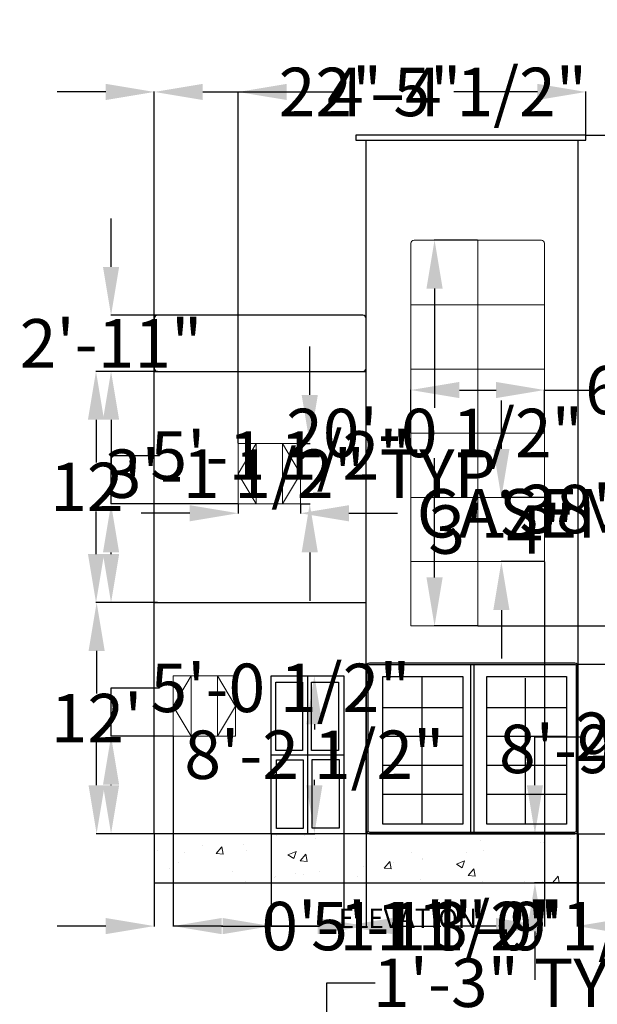
# Model space of a CAD drawing. Units: inches. Extents: x 7323 to 9737, y 2037 to 3322.
# Tile 17 of 19: x 8562 to 8922, y 2709 to 3322. Entities that reach past the tile are written whole.
import ezdxf

# ---------------------------------------------------------------- set-up
doc = ezdxf.new("R2010")
doc.units = ezdxf.units.IN
doc.header["$MEASUREMENT"] = 0
for name, color, linetype, lineweight in [('A-ANNO-DIMS', 2, 'Continuous', 18), ('A-ANNO-TEXT', 7, 'Continuous', 25), ('A-DOOR', 4, 'Continuous', 25), ('A-ELEV', 7, 'Continuous', 30), ('A-GLAZ', 4, 'Continuous', 18), ('A-ROOF', 7, 'Continuous', 30)]:
    doc.layers.add(name, color=color, linetype=linetype, lineweight=lineweight)
doc.layers.add('A-ELEV-PATT', color=32, linetype='Continuous', lineweight=13, true_color=0xcd6928)
doc.styles.get("Standard").update_dxf_attribs({"font": 'arial.ttf'})
doc.dimstyles.get("Standard").update_dxf_attribs({"dimtxt": 30.18, "dimasz": 30.18, "dimexe": 0.18, "dimexo": 0.0625, "dimgap": 0.09, "dimtad": 0, "dimtih": 1, "dimtoh": 1, "dimdec": 0, "dimzin": 0, "dimdsep": 46, "dimlunit": 3, "dimtxsty": 'Standard', "dimcen": 0.09, "dimadec": 0, "dimazin": 0, "dimtfac": 1, "dimtdec": 0, "dimtofl": 0, "dimtmove": 0, "dimatfit": 3, "dimfxl": 1, "dimtolj": 1, "dimtzin": 0, "dimarcsym": 0})

# ---------------------------------------------------------------- blocks, each defined once
blk = doc.blocks.new('*D5')
at = {"layer": 'A-ANNO-DIMS', "color": 0, "lineweight": -2, "transparency": 16777216}
for p, q in [((8646.01, 2959.19), (8610, 2959.19)), ((8610.18, 2929.01), (8610.18, 2902.43)), ((8610.18, 2845.37), (8610.18, 2871.95)), ((8646.01, 2815.19), (8610, 2815.19))]:
    blk.add_line(p, q, dxfattribs=at)
at = {"layer": 'A-ANNO-DIMS', "color": 0, "transparency": 16777216}
for points in [[(8605.15, 2929.01), (8615.21, 2929.01), (8610.18, 2959.19)], [(8605.15, 2845.37), (8615.21, 2845.37), (8610.18, 2815.19)]]:
    blk.add_solid(points, dxfattribs=at)
at = {"layer": 'Defpoints', "color": 0, "transparency": 16777216}
for p in [(8610.18, 2959.19), (8646.07, 2959.19), (8646.07, 2815.19)]:
    blk.add_point(p, dxfattribs=at)
at = {"layer": 'A-ANNO-DIMS', "color": 0, "transparency": 16777216, "insert": (8610.18, 2887.19), "char_height": 30.18, "attachment_point": 5}
blk.add_mtext("\\A1;12'", dxfattribs=at)
blk = doc.blocks.new('*D6')
at = {"layer": 'A-ANNO-DIMS', "color": 0, "lineweight": -2, "transparency": 16777216}
for p, q in [((8648.01, 3103.19), (8609.62, 3103.19)), ((8609.8, 3073.01), (8609.8, 3046.43)), ((8609.8, 2989.37), (8609.8, 3015.95)), ((8648.01, 2959.19), (8609.62, 2959.19))]:
    blk.add_line(p, q, dxfattribs=at)
at = {"layer": 'A-ANNO-DIMS', "color": 0, "transparency": 16777216}
for points in [[(8604.77, 3073.01), (8614.83, 3073.01), (8609.8, 3103.19)], [(8604.77, 2989.37), (8614.83, 2989.37), (8609.8, 2959.19)]]:
    blk.add_solid(points, dxfattribs=at)
at = {"layer": 'Defpoints', "color": 0, "transparency": 16777216}
for p in [(8648.07, 3103.19), (8609.8, 2959.19), (8648.07, 2959.19)]:
    blk.add_point(p, dxfattribs=at)
at = {"layer": 'A-ANNO-DIMS', "color": 0, "transparency": 16777216, "insert": (8609.8, 3031.19), "char_height": 30.18, "attachment_point": 5}
blk.add_mtext("\\A1;12'", dxfattribs=at)
blk = doc.blocks.new('WIN-ELEV-CASEMENT')
for p, q in [((11.18, 37.71), (0, 18.85)), ((11.18, 37.71), (11.18, 0)), ((27.64, 37.71), (27.64, 0)), ((27.64, 37.71), (38.77, 18.85)), ((0, 18.85), (11.18, 0)), ((38.77, 18.85), (27.64, 0))]:
    blk.add_line(p, q)
blk.add_lwpolyline([(38.77, 37.71), (38.77, 37.71), (0, 37.71), (0, 37.71), (0, 0), (0, 0), (38.77, 0), (38.77, 0)], close=True)
blk = doc.blocks.new('*D45')
at = {"layer": 'A-ANNO-DIMS', "color": 0, "lineweight": -2, "transparency": 16777216}
for p, q in [((8725.79, 2664.36), (8695.61, 2664.36)), ((8755.97, 2662.02), (8755.97, 2664.54)), ((8772, 2662.02), (8772, 2664.54)), ((8802.18, 2664.36), (8832.36, 2664.36))]:
    blk.add_line(p, q, dxfattribs=at)
at = {"layer": 'A-ANNO-DIMS', "color": 0, "transparency": 16777216}
for points in [[(8725.79, 2669.39), (8725.79, 2659.33), (8755.97, 2664.36)], [(8802.18, 2669.39), (8802.18, 2659.33), (8772, 2664.36)]]:
    blk.add_solid(points, dxfattribs=at)
at = {"layer": 'Defpoints', "color": 0, "transparency": 16777216}
for p in [(8755.97, 2661.96), (8772, 2664.36), (8772, 2661.96)]:
    blk.add_point(p, dxfattribs=at)
at = {"layer": 'A-ANNO-DIMS', "color": 0, "transparency": 16777216, "insert": (9094.8, 2664.36), "char_height": 30.18, "attachment_point": 5}
blk.add_mtext('\\A1;BEDSIDE TABLE 1\'-4" TYP.', dxfattribs=at)
blk = doc.blocks.new('*D46')
at = {"layer": 'A-ANNO-DIMS', "color": 0, "lineweight": -2, "transparency": 16777216}
for p, q in [((8753.57, 2692.14), (8753.57, 2722.32)), ((8753.57, 2722.32), (8783.75, 2722.32)), ((8755.91, 2661.96), (8753.39, 2661.96)), ((8755.91, 2647.12), (8753.39, 2647.12)), ((8753.57, 2616.94), (8753.57, 2586.76))]:
    blk.add_line(p, q, dxfattribs=at)
at = {"layer": 'A-ANNO-DIMS', "color": 0, "transparency": 16777216}
for points in [[(8748.54, 2692.14), (8758.6, 2692.14), (8753.57, 2661.96)], [(8748.54, 2616.94), (8758.6, 2616.94), (8753.57, 2647.12)]]:
    blk.add_solid(points, dxfattribs=at)
at = {"layer": 'Defpoints', "color": 0, "transparency": 16777216}
for p in [(8753.57, 2661.96), (8755.97, 2661.96), (8755.97, 2647.12)]:
    blk.add_point(p, dxfattribs=at)
at = {"layer": 'A-ANNO-DIMS', "color": 0, "transparency": 16777216, "insert": (8874.4, 2722.32), "char_height": 30.18, "attachment_point": 5}
blk.add_mtext('\\A1;1\'-3" TYP.', dxfattribs=at)
blk = doc.blocks.new('*D57')
at = {"layer": 'A-ANNO-DIMS', "color": 0, "lineweight": -2, "transparency": 16777216}
for p, q in [((8698.34, 3020.54), (8698.34, 3014.6)), ((8737.11, 3020.54), (8737.11, 3014.6)), ((8668.16, 3014.78), (8637.98, 3014.78)), ((8767.29, 3014.78), (8797.47, 3014.78))]:
    blk.add_line(p, q, dxfattribs=at)
at = {"layer": 'A-ANNO-DIMS', "color": 0, "transparency": 16777216}
for points in [[(8668.16, 3019.81), (8668.16, 3009.75), (8698.34, 3014.78)], [(8767.29, 3019.81), (8767.29, 3009.75), (8737.11, 3014.78)]]:
    blk.add_solid(points, dxfattribs=at)
at = {"layer": 'Defpoints', "color": 0, "transparency": 16777216}
for p in [(8698.34, 3020.6), (8737.11, 3020.6), (8737.11, 3014.78)]:
    blk.add_point(p, dxfattribs=at)
at = {"layer": 'A-ANNO-DIMS', "color": 0, "transparency": 16777216, "insert": (9012.35, 3014.78), "char_height": 30.18, "attachment_point": 5}
blk.add_mtext('\\A1;CASEMENT 3\'-3" TYP.', dxfattribs=at)
blk = doc.blocks.new('*D58')
at = {"layer": 'A-ANNO-DIMS', "color": 0, "lineweight": -2, "transparency": 16777216}
for p, q in [((8742.92, 3088.49), (8742.92, 3118.67)), ((8737.17, 3058.31), (8743.1, 3058.31)), ((8737.17, 3020.6), (8743.1, 3020.6)), ((8742.92, 2990.42), (8742.92, 2960.24))]:
    blk.add_line(p, q, dxfattribs=at)
at = {"layer": 'A-ANNO-DIMS', "color": 0, "transparency": 16777216}
for points in [[(8737.89, 3088.49), (8747.95, 3088.49), (8742.92, 3058.31)], [(8737.89, 2990.42), (8747.95, 2990.42), (8742.92, 3020.6)]]:
    blk.add_solid(points, dxfattribs=at)
at = {"layer": 'Defpoints', "color": 0, "transparency": 16777216}
for p in [(8737.11, 3058.31), (8742.92, 3058.31), (8737.11, 3020.6)]:
    blk.add_point(p, dxfattribs=at)
at = {"layer": 'A-ANNO-DIMS', "color": 0, "transparency": 16777216, "insert": (8742.92, 3039.45), "char_height": 30.18, "attachment_point": 5}
blk.add_mtext('\\A1;3\'-1 1/2" TYP.', dxfattribs=at)
blk = doc.blocks.new('*D82')
at = {"layer": 'A-ANNO-DIMS', "color": 0, "lineweight": -2, "transparency": 16777216}
for p, q in [((8646.07, 3103.25), (8646.07, 3277.41)), ((8676.25, 3277.23), (8728.3, 3277.23)), ((8884.72, 3277.23), (8832.67, 3277.23)), ((8914.9, 3250.4), (8914.9, 3277.41))]:
    blk.add_line(p, q, dxfattribs=at)
at = {"layer": 'A-ANNO-DIMS', "color": 0, "transparency": 16777216}
for points in [[(8676.25, 3282.26), (8676.25, 3272.2), (8646.07, 3277.23)], [(8884.72, 3282.26), (8884.72, 3272.2), (8914.9, 3277.23)]]:
    blk.add_solid(points, dxfattribs=at)
at = {"layer": 'Defpoints', "color": 0, "transparency": 16777216}
for p in [(8914.9, 3277.23), (8914.9, 3250.33), (8646.07, 3103.19)]:
    blk.add_point(p, dxfattribs=at)
at = {"layer": 'A-ANNO-DIMS', "color": 0, "transparency": 16777216, "insert": (8780.48, 3277.23), "char_height": 30.18, "attachment_point": 5}
blk.add_mtext('\\A1;22\'-5"', dxfattribs=at)
blk = doc.blocks.new('*D83')
at = {"layer": 'A-ANNO-DIMS', "color": 0, "lineweight": -2, "transparency": 16777216}
for p, q in [((8914.96, 3250.33), (8941.98, 3250.33)), ((8941.8, 3220.15), (8941.8, 3032.95)), ((8941.8, 2814.72), (8941.8, 3001.93)), ((8910.13, 2784.54), (8941.98, 2784.54))]:
    blk.add_line(p, q, dxfattribs=at)
at = {"layer": 'A-ANNO-DIMS', "color": 0, "transparency": 16777216}
for points in [[(8936.77, 3220.15), (8946.83, 3220.15), (8941.8, 3250.33)], [(8936.77, 2814.72), (8946.83, 2814.72), (8941.8, 2784.54)]]:
    blk.add_solid(points, dxfattribs=at)
at = {"layer": 'Defpoints', "color": 0, "transparency": 16777216}
for p in [(8914.9, 3250.33), (8941.8, 3250.33), (8910.07, 2784.54)]:
    blk.add_point(p, dxfattribs=at)
at = {"layer": 'A-ANNO-DIMS', "color": 0, "transparency": 16777216, "insert": (8941.8, 3017.44), "char_height": 30.18, "attachment_point": 5}
blk.add_mtext('\\A1;38\'-10"', dxfattribs=at)
blk = doc.blocks.new('*D84')
at = {"layer": 'A-ANNO-DIMS', "color": 0, "lineweight": -2, "transparency": 16777216}
for p, q in [((8778.071366, 2815.126036), (8778.071366, 2757.459848)), ((8910.071366, 2815.126036), (8910.071366, 2757.459848)), ((8747.891366, 2757.639848), (8717.711366, 2757.639848)), ((8940.251366, 2757.639848), (8970.431366, 2757.639848))]:
    blk.add_line(p, q, dxfattribs=at)
at = {"layer": 'A-ANNO-DIMS', "color": 0, "transparency": 16777216}
for points in [[(8747.891366, 2762.669848), (8747.891366, 2752.609848), (8778.071366, 2757.639848)], [(8940.251366, 2762.669848), (8940.251366, 2752.609848), (8910.071366, 2757.639848)]]:
    blk.add_solid(points, dxfattribs=at)
at = {"layer": 'Defpoints', "color": 0, "transparency": 16777216}
for p in [(8778.071366, 2815.188536), (8910.071366, 2815.188536), (8910.071366, 2757.639848)]:
    blk.add_point(p, dxfattribs=at)
at = {"layer": 'A-ANNO-DIMS', "color": 0, "transparency": 16777216, "insert": (8844.071366, 2757.639848), "char_height": 30.18, "attachment_point": 5}
blk.add_mtext('\\A1;11\'-0"', dxfattribs=at)
blk = doc.blocks.new('*D85')
at = {"layer": 'A-ANNO-DIMS', "color": 0, "lineweight": -2, "transparency": 16777216}
for p, q in [((8805.94, 3064.71), (8805.94, 3091.73)), ((8836.12, 3091.55), (8858.99, 3091.55)), ((8889.17, 3064.71), (8889.17, 3091.73)), ((8889.17, 3091.55), (8919.35, 3091.55))]:
    blk.add_line(p, q, dxfattribs=at)
at = {"layer": 'A-ANNO-DIMS', "color": 0, "transparency": 16777216}
for points in [[(8836.12, 3096.58), (8836.12, 3086.52), (8805.94, 3091.55)], [(8858.99, 3096.58), (8858.99, 3086.52), (8889.17, 3091.55)]]:
    blk.add_solid(points, dxfattribs=at)
at = {"layer": 'Defpoints', "color": 0, "transparency": 16777216}
for p in [(8889.17, 3091.55), (8805.94, 3064.65), (8889.17, 3064.65)]:
    blk.add_point(p, dxfattribs=at)
at = {"layer": 'A-ANNO-DIMS', "color": 0, "transparency": 16777216, "insert": (8971.36, 3091.55), "char_height": 30.18, "attachment_point": 5}
blk.add_mtext('\\A1;6\'-11"', dxfattribs=at)
blk = doc.blocks.new('*D86')
at = {"layer": 'A-ANNO-DIMS', "color": 0, "lineweight": -2, "transparency": 16777216}
for p, q in [((8847.49, 3184.93), (8820.47, 3184.93)), ((8820.65, 3154.75), (8820.65, 3080.48)), ((8820.65, 2974.83), (8820.65, 3049.09)), ((8847.49, 2944.65), (8820.47, 2944.65))]:
    blk.add_line(p, q, dxfattribs=at)
at = {"layer": 'A-ANNO-DIMS', "color": 0, "transparency": 16777216}
for points in [[(8815.62, 3154.75), (8825.68, 3154.75), (8820.65, 3184.93)], [(8815.62, 2974.83), (8825.68, 2974.83), (8820.65, 2944.65)]]:
    blk.add_solid(points, dxfattribs=at)
at = {"layer": 'Defpoints', "color": 0, "transparency": 16777216}
for p in [(8820.65, 3184.93), (8847.55, 3184.93), (8847.55, 2944.65)]:
    blk.add_point(p, dxfattribs=at)
at = {"layer": 'A-ANNO-DIMS', "color": 0, "transparency": 16777216, "insert": (8820.65, 3064.79), "char_height": 30.18, "attachment_point": 5}
blk.add_mtext('\\A1;20\'-0 1/2"', dxfattribs=at)
blk = doc.blocks.new('*D87')
at = {"layer": 'A-ANNO-DIMS', "color": 0, "lineweight": -2, "transparency": 16777216}
for p, q in [((8619.17, 2875.84), (8619.17, 2906.02)), ((8619.17, 2906.02), (8649.35, 2906.02)), ((8657.74, 2875.84), (8618.99, 2875.84)), ((8619.17, 2845.37), (8619.17, 2845.66)), ((8646.01, 2815.19), (8618.99, 2815.19))]:
    blk.add_line(p, q, dxfattribs=at)
at = {"layer": 'A-ANNO-DIMS', "color": 0, "transparency": 16777216}
for points in [[(8614.14, 2845.66), (8624.2, 2845.66), (8619.17, 2875.84)], [(8614.14, 2845.37), (8624.2, 2845.37), (8619.17, 2815.19)]]:
    blk.add_solid(points, dxfattribs=at)
at = {"layer": 'Defpoints', "color": 0, "transparency": 16777216}
for p in [(8619.17, 2875.84), (8657.81, 2875.84), (8646.07, 2815.19)]:
    blk.add_point(p, dxfattribs=at)
at = {"layer": 'A-ANNO-DIMS', "color": 0, "transparency": 16777216, "insert": (8724.72, 2906.02), "char_height": 30.18, "attachment_point": 5}
blk.add_mtext('\\A1;5\'-0 1/2"', dxfattribs=at)
blk = doc.blocks.new('*D88')
at = {"layer": 'A-ANNO-DIMS', "color": 0, "lineweight": -2, "transparency": 16777216}
for p, q in [((8941.797746, 2974.828285), (8941.797746, 3005.008285)), ((8941.797746, 3005.008285), (8971.977746, 3005.008285)), ((8847.615005, 2944.648285), (8941.977746, 2944.648285)), ((8909.54808, 2920.815964), (8941.977746, 2920.815964)), ((8941.797746, 2890.635964), (8941.797746, 2860.455964))]:
    blk.add_line(p, q, dxfattribs=at)
at = {"layer": 'A-ANNO-DIMS', "color": 0, "transparency": 16777216}
for points in [[(8936.767746, 2974.828285), (8946.827746, 2974.828285), (8941.797746, 2944.648285)], [(8936.767746, 2890.635964), (8946.827746, 2890.635964), (8941.797746, 2920.815964)]]:
    blk.add_solid(points, dxfattribs=at)
at = {"layer": 'Defpoints', "color": 0, "transparency": 16777216}
for p in [(8847.552505, 2944.648285), (8941.797746, 2944.648285), (8909.48558, 2920.815964)]:
    blk.add_point(p, dxfattribs=at)
at = {"layer": 'A-ANNO-DIMS', "color": 0, "transparency": 16777216, "insert": (9012.438128, 3005.008285), "char_height": 30.18, "attachment_point": 5}
blk.add_mtext('\\A1;2\'-0"', dxfattribs=at)
blk = doc.blocks.new('*D89')
at = {"layer": 'A-ANNO-DIMS', "color": 0, "lineweight": -2, "transparency": 16777216}
for p, q in [((8657.81, 2875.78), (8657.81, 2757.46)), ((8718.91, 2815.13), (8718.91, 2757.46)), ((8687.99, 2757.64), (8688.73, 2757.64)), ((8718.91, 2757.64), (8749.09, 2757.64))]:
    blk.add_line(p, q, dxfattribs=at)
at = {"layer": 'A-ANNO-DIMS', "color": 0, "transparency": 16777216}
for points in [[(8687.99, 2762.67), (8687.99, 2752.61), (8657.81, 2757.64)], [(8688.73, 2762.67), (8688.73, 2752.61), (8718.91, 2757.64)]]:
    blk.add_solid(points, dxfattribs=at)
at = {"layer": 'Defpoints', "color": 0, "transparency": 16777216}
for p in [(8657.81, 2875.84), (8718.91, 2815.19), (8718.91, 2757.64)]:
    blk.add_point(p, dxfattribs=at)
at = {"layer": 'A-ANNO-DIMS', "color": 0, "transparency": 16777216, "insert": (8789.29, 2757.64), "char_height": 30.18, "attachment_point": 5}
blk.add_mtext('\\A1;5\'-1"', dxfattribs=at)
blk = doc.blocks.new('*D90')
at = {"layer": 'A-ANNO-DIMS', "color": 0, "lineweight": -2, "transparency": 16777216}
for p, q in [((8718.91, 2815.13), (8718.91, 2757.46)), ((8764.24, 2815.13), (8764.24, 2757.46)), ((8688.73, 2757.64), (8658.55, 2757.64)), ((8794.42, 2757.64), (8824.6, 2757.64))]:
    blk.add_line(p, q, dxfattribs=at)
at = {"layer": 'A-ANNO-DIMS', "color": 0, "transparency": 16777216}
for points in [[(8688.73, 2762.67), (8688.73, 2752.61), (8718.91, 2757.64)], [(8794.42, 2762.67), (8794.42, 2752.61), (8764.24, 2757.64)]]:
    blk.add_solid(points, dxfattribs=at)
at = {"layer": 'Defpoints', "color": 0, "transparency": 16777216}
for p in [(8718.91, 2815.19), (8764.24, 2815.19), (8764.24, 2757.64)]:
    blk.add_point(p, dxfattribs=at)
at = {"layer": 'A-ANNO-DIMS', "color": 0, "transparency": 16777216, "insert": (8899.95, 2757.64), "char_height": 30.18, "attachment_point": 5}
blk.add_mtext('\\A1;3\'-9 1/2"', dxfattribs=at)
blk = doc.blocks.new('*D91')
at = {"layer": 'A-ANNO-DIMS', "color": 0, "lineweight": -2, "transparency": 16777216}
for p, q in [((8909.55, 2920.82), (8941.98, 2920.82)), ((8941.8, 2890.64), (8941.8, 2883.7)), ((8941.8, 2845.37), (8941.8, 2852.31)), ((8910.13, 2815.19), (8941.98, 2815.19))]:
    blk.add_line(p, q, dxfattribs=at)
at = {"layer": 'A-ANNO-DIMS', "color": 0, "transparency": 16777216}
for points in [[(8936.77, 2890.64), (8946.83, 2890.64), (8941.8, 2920.82)], [(8936.77, 2845.37), (8946.83, 2845.37), (8941.8, 2815.19)]]:
    blk.add_solid(points, dxfattribs=at)
at = {"layer": 'Defpoints', "color": 0, "transparency": 16777216}
for p in [(8909.49, 2920.82), (8941.8, 2920.82), (8910.07, 2815.19)]:
    blk.add_point(p, dxfattribs=at)
at = {"layer": 'A-ANNO-DIMS', "color": 0, "transparency": 16777216, "insert": (8941.8, 2868), "char_height": 30.18, "attachment_point": 5}
blk.add_mtext('\\A1;8\'-9 1/2"', dxfattribs=at)
blk = doc.blocks.new('*D92')
at = {"layer": 'A-ANNO-DIMS', "color": 0, "lineweight": -2, "transparency": 16777216}
for p, q in [((8883.17, 2845.37), (8883.17, 2875.55)), ((8883.17, 2875.55), (8913.35, 2875.55)), ((8910.01, 2815.19), (8882.99, 2815.19)), ((8910.01, 2784.54), (8882.99, 2784.54)), ((8883.17, 2754.36), (8883.17, 2724.18))]:
    blk.add_line(p, q, dxfattribs=at)
at = {"layer": 'A-ANNO-DIMS', "color": 0, "transparency": 16777216}
for points in [[(8878.14, 2845.37), (8888.2, 2845.37), (8883.17, 2815.19)], [(8878.14, 2754.36), (8888.2, 2754.36), (8883.17, 2784.54)]]:
    blk.add_solid(points, dxfattribs=at)
at = {"layer": 'Defpoints', "color": 0, "transparency": 16777216}
for p in [(8883.17, 2815.19), (8910.07, 2815.19), (8910.07, 2784.54)]:
    blk.add_point(p, dxfattribs=at)
at = {"layer": 'A-ANNO-DIMS', "color": 0, "transparency": 16777216, "insert": (8988.97, 2875.55), "char_height": 30.18, "attachment_point": 5}
blk.add_mtext('\\A1;2\'-6 1/2"', dxfattribs=at)
blk = doc.blocks.new('*D101')
at = {"layer": 'A-ANNO-DIMS', "color": 0, "lineweight": -2, "transparency": 16777216}
for p, q in [((8889.17, 2984.59), (8889.17, 2757.46)), ((8909.49, 2920.75), (8909.49, 2757.46)), ((8858.99, 2757.64), (8828.81, 2757.64)), ((8939.67, 2757.64), (8969.85, 2757.64))]:
    blk.add_line(p, q, dxfattribs=at)
at = {"layer": 'A-ANNO-DIMS', "color": 0, "transparency": 16777216}
for points in [[(8858.99, 2762.67), (8858.99, 2752.61), (8889.17, 2757.64)], [(8939.67, 2762.67), (8939.67, 2752.61), (8909.49, 2757.64)]]:
    blk.add_solid(points, dxfattribs=at)
at = {"layer": 'Defpoints', "color": 0, "transparency": 16777216}
for p in [(8889.17, 2984.65), (8909.49, 2920.82), (8909.49, 2757.64)]:
    blk.add_point(p, dxfattribs=at)
at = {"layer": 'A-ANNO-DIMS', "color": 0, "transparency": 16777216, "insert": (9043.79, 2757.64), "char_height": 30.18, "attachment_point": 5}
blk.add_mtext('\\A1;1\'-8 1/2"', dxfattribs=at)
blk = doc.blocks.new('*D102')
at = {"layer": 'A-ANNO-DIMS', "color": 0, "lineweight": -2, "transparency": 16777216}
for p, q in [((8619.171366, 3168.286532), (8619.171366, 3198.466532)), ((8648.008866, 3138.106532), (8618.991366, 3138.106532)), ((8646.008866, 3103.188536), (8618.991366, 3103.188536)), ((8619.171366, 3073.008536), (8619.171366, 3042.828536))]:
    blk.add_line(p, q, dxfattribs=at)
at = {"layer": 'A-ANNO-DIMS', "color": 0, "transparency": 16777216}
for points in [[(8614.141366, 3168.286532), (8624.201366, 3168.286532), (8619.171366, 3138.106532)], [(8614.141366, 3073.008536), (8624.201366, 3073.008536), (8619.171366, 3103.188536)]]:
    blk.add_solid(points, dxfattribs=at)
at = {"layer": 'Defpoints', "color": 0, "transparency": 16777216}
for p in [(8619.171366, 3138.106532), (8648.071366, 3138.106532), (8646.071366, 3103.188536)]:
    blk.add_point(p, dxfattribs=at)
at = {"layer": 'A-ANNO-DIMS', "color": 0, "transparency": 16777216, "insert": (8619.171366, 3120.647534), "char_height": 30.18, "attachment_point": 5}
blk.add_mtext('\\A1;2\'-11"', dxfattribs=at)
blk = doc.blocks.new('*D117')
at = {"layer": 'A-ANNO-DIMS', "color": 0, "lineweight": -2, "transparency": 16777216}
for p, q in [((8862.269216, 3054.828285), (8862.269216, 3085.008285)), ((8889.106716, 3024.648285), (8862.089216, 3024.648285)), ((8889.106716, 2984.648285), (8862.089216, 2984.648285)), ((8862.269216, 2954.468285), (8862.269216, 2924.288285))]:
    blk.add_line(p, q, dxfattribs=at)
at = {"layer": 'A-ANNO-DIMS', "color": 0, "transparency": 16777216}
for points in [[(8857.239216, 3054.828285), (8867.299216, 3054.828285), (8862.269216, 3024.648285)], [(8857.239216, 2954.468285), (8867.299216, 2954.468285), (8862.269216, 2984.648285)]]:
    blk.add_solid(points, dxfattribs=at)
at = {"layer": 'Defpoints', "color": 0, "transparency": 16777216}
for p in [(8862.269216, 3024.648285), (8889.169216, 3024.648285), (8889.169216, 2984.648285)]:
    blk.add_point(p, dxfattribs=at)
at = {"layer": 'A-ANNO-DIMS', "color": 0, "transparency": 16777216, "insert": (8862.269216, 3004.648285), "char_height": 30.18, "attachment_point": 5}
blk.add_mtext('\\A1;3\'-4"', dxfattribs=at)
blk = doc.blocks.new('*D118')
at = {"layer": 'A-ANNO-DIMS', "color": 0, "lineweight": -2, "transparency": 16777216}
for p, q in [((8718.97, 2913.55), (8745.99, 2913.55)), ((8745.81, 2883.37), (8745.81, 2880.06)), ((8745.81, 2845.37), (8745.81, 2848.67)), ((8718.97, 2815.19), (8745.99, 2815.19))]:
    blk.add_line(p, q, dxfattribs=at)
at = {"layer": 'A-ANNO-DIMS', "color": 0, "transparency": 16777216}
for points in [[(8740.78, 2883.37), (8750.84, 2883.37), (8745.81, 2913.55)], [(8740.78, 2845.37), (8750.84, 2845.37), (8745.81, 2815.19)]]:
    blk.add_solid(points, dxfattribs=at)
at = {"layer": 'Defpoints', "color": 0, "transparency": 16777216}
for p in [(8718.91, 2913.55), (8718.91, 2815.19), (8745.81, 2815.19)]:
    blk.add_point(p, dxfattribs=at)
at = {"layer": 'A-ANNO-DIMS', "color": 0, "transparency": 16777216, "insert": (8745.81, 2864.37), "char_height": 30.18, "attachment_point": 5}
blk.add_mtext('\\A1;8\'-2 1/2"', dxfattribs=at)
blk = doc.blocks.new('*D119')
at = {"layer": 'A-ANNO-DIMS', "color": 0, "lineweight": -2, "transparency": 16777216}
for p, q in [((8619.17, 3020.6), (8619.17, 3050.78)), ((8619.17, 3050.78), (8649.35, 3050.78)), ((8698.27, 3020.6), (8618.99, 3020.6)), ((8619.17, 2989.37), (8619.17, 2990.42)), ((8646.01, 2959.19), (8618.99, 2959.19))]:
    blk.add_line(p, q, dxfattribs=at)
at = {"layer": 'A-ANNO-DIMS', "color": 0, "transparency": 16777216}
for points in [[(8614.14, 2990.42), (8624.2, 2990.42), (8619.17, 3020.6)], [(8614.14, 2989.37), (8624.2, 2989.37), (8619.17, 2959.19)]]:
    blk.add_solid(points, dxfattribs=at)
at = {"layer": 'Defpoints', "color": 0, "transparency": 16777216}
for p in [(8619.17, 3020.6), (8698.34, 3020.6), (8646.07, 2959.19)]:
    blk.add_point(p, dxfattribs=at)
at = {"layer": 'A-ANNO-DIMS', "color": 0, "transparency": 16777216, "insert": (8724.72, 3050.78), "char_height": 30.18, "attachment_point": 5}
blk.add_mtext('\\A1;5\'-1 1/2"', dxfattribs=at)
blk = doc.blocks.new('*D120')
at = {"layer": 'A-ANNO-DIMS', "color": 0, "lineweight": -2, "transparency": 16777216}
for p, q in [((8615.89, 3277.23), (8585.71, 3277.23)), ((8646.07, 3103.25), (8646.07, 3277.41)), ((8698.34, 3058.37), (8698.34, 3277.41)), ((8728.52, 3277.23), (8758.7, 3277.23))]:
    blk.add_line(p, q, dxfattribs=at)
at = {"layer": 'A-ANNO-DIMS', "color": 0, "transparency": 16777216}
for points in [[(8615.89, 3282.26), (8615.89, 3272.2), (8646.07, 3277.23)], [(8728.52, 3282.26), (8728.52, 3272.2), (8698.34, 3277.23)]]:
    blk.add_solid(points, dxfattribs=at)
at = {"layer": 'Defpoints', "color": 0, "transparency": 16777216}
for p in [(8698.34, 3277.23), (8646.07, 3103.19), (8698.34, 3058.31)]:
    blk.add_point(p, dxfattribs=at)
at = {"layer": 'A-ANNO-DIMS', "color": 0, "transparency": 16777216, "insert": (8834.67, 3277.23), "char_height": 30.18, "attachment_point": 5}
blk.add_mtext('\\A1;4\'-4 1/2"', dxfattribs=at)
blk = doc.blocks.new('*D121')
at = {"layer": 'A-ANNO-DIMS', "color": 0, "lineweight": -2, "transparency": 16777216}
for p, q in [((8657.81, 2875.78), (8657.81, 2757.46)), ((8646.07, 2815.13), (8646.07, 2757.46)), ((8615.89, 2757.64), (8585.71, 2757.64)), ((8687.99, 2757.64), (8718.17, 2757.64))]:
    blk.add_line(p, q, dxfattribs=at)
at = {"layer": 'A-ANNO-DIMS', "color": 0, "transparency": 16777216}
for points in [[(8615.89, 2762.67), (8615.89, 2752.61), (8646.07, 2757.64)], [(8687.99, 2762.67), (8687.99, 2752.61), (8657.81, 2757.64)]]:
    blk.add_solid(points, dxfattribs=at)
at = {"layer": 'Defpoints', "color": 0, "transparency": 16777216}
for p in [(8657.81, 2875.84), (8646.07, 2815.19), (8657.81, 2757.64)]:
    blk.add_point(p, dxfattribs=at)
at = {"layer": 'A-ANNO-DIMS', "color": 0, "transparency": 16777216, "insert": (8805.25, 2757.64), "char_height": 30.18, "attachment_point": 5}
blk.add_mtext('\\A1;0\'-11 1/2"', dxfattribs=at)

msp = doc.modelspace()

# ---------------------------------------------------------------- hatches: boundary and pattern name
at = {"layer": 'A-ELEV-PATT'}
h = msp.add_hatch(dxfattribs=at)
h.set_pattern_fill('AR-CONC', color=256, scale=7.3)
h.set_pattern_definition([(50, (294.767, -28.717), (52.36, -4.5809), [5.475, -60.225]), (355, (294.767, -28.717), (-10.12885, 54.91003), [4.38, -48.18]), (100.45144, (299.13, -29.1), (42.23115, 50.32912), [4.65303, -51.18337]), (46.1842, (294.77, -14.12), (77.9086, -12.0829), [8.2125, -90.3375]), (96.6356, (301.26, -15.124), (68.2303, 71.11066), [6.97955, -76.7751]), (351.1842, (294.77, -14.12), (68.2303, 71.11066), [6.57, -72.27]), (21, (302.067, -17.767), (43.57421, -29.39118), [5.475, -60.225]), (326, (302.067, -17.767), (17.76202, 52.93595), [4.38, -48.18]), (71.45144, (305.7, -20.216), (61.33623, 23.54477), [4.65303, -51.18337]), (37.5, (294.767, -28.717), (0.88767, 24.30125), [0, -47.596, 0, -48.91, 0, -48.3625]), (7.5, (294.767, -28.717), (19.204076, 28.792055), [0, -27.886, 0, -46.501, 0, -18.4325]), (327.5, (278.488, -28.717), (38.969038, -1.646506), [0, -18.25, 0, -56.94, 0, -75.555]), (317.5, (271.188, -28.717), (42.57259, 7.30766), [0, -23.725, 0, -37.814, 0, -53.655])])
h.paths.add_polyline_path([(8646.07, 2815.19), (8646.07, 2784.54), (8910.07, 2784.54), (8910.07, 2815.19)])

# ---------------------------------------------------------------- linework, layer by layer
at = {"layer": 'A-DOOR'}
for p, q in [((8843.07, 2920.4), (8843.07, 2816.19)), ((8845.07, 2920.4), (8845.07, 2816.19)), ((8741.57, 2913.55), (8741.57, 2815.19)), ((8812.69, 2913.17), (8812.69, 2821.58)), ((8877.09, 2912.17), (8877.09, 2821.58)), ((8788.53, 2893.84), (8838.23, 2893.84)), ((8853.14, 2893.84), (8902.74, 2893.84)), ((8788.53, 2875.84), (8838.34, 2875.84)), ((8853.14, 2875.84), (8902.74, 2875.84)), ((8718.91, 2864.37), (8764.24, 2864.37)), ((8788.53, 2857.84), (8838.34, 2857.84)), ((8853.14, 2857.84), (8902.74, 2857.84)), ((8788.53, 2839.84), (8838.34, 2839.84)), ((8853.14, 2839.84), (8902.74, 2839.84))]:
    msp.add_line(p, q, dxfattribs=at)
for points in [[(8778.07, 2817.19, 0.414214), (8780.07, 2815.19), (8908.07, 2815.19, 0.414214), (8910.07, 2817.19), (8910.07, 2919.4, 0.414214), (8908.07, 2921.4), (8780.07, 2921.4, 0.414214), (8778.07, 2919.4)], [(8779.07, 2817.19, 0.414214), (8780.07, 2816.19), (8908.07, 2816.19, 0.414214), (8909.07, 2817.19), (8909.07, 2919.4, 0.414214), (8908.07, 2920.4), (8780.07, 2920.4, 0.414214), (8779.07, 2919.4)]]:
    msp.add_lwpolyline(points, format="xyb", close=True, dxfattribs=at)
for points in [[(8764.24, 2815.19), (8764.24, 2815.19), (8718.91, 2815.19), (8718.91, 2815.19), (8718.91, 2913.55), (8718.91, 2913.55), (8764.24, 2913.55), (8764.24, 2913.55)], [(8721.72, 2909.56), (8721.72, 2909.56), (8738.48, 2909.56), (8738.48, 2909.56), (8738.48, 2866.92), (8738.48, 2866.92), (8721.72, 2866.92), (8721.72, 2866.92)], [(8744.06, 2909.56), (8744.06, 2909.56), (8760.82, 2909.56), (8760.82, 2909.56), (8760.82, 2866.92), (8760.82, 2866.92), (8744.06, 2866.92), (8744.06, 2866.92)], [(8788.53, 2913.17), (8788.53, 2913.17), (8838.23, 2913.17), (8838.23, 2913.17), (8838.23, 2821.2), (8838.23, 2821.2), (8788.53, 2821.2), (8788.53, 2821.2)], [(8853.14, 2913.17), (8853.14, 2913.17), (8902.84, 2913.17), (8902.84, 2913.17), (8902.84, 2821.2), (8902.84, 2821.2), (8853.14, 2821.2), (8853.14, 2821.2)], [(8722.17, 2861.16), (8722.17, 2861.16), (8738.92, 2861.16), (8738.92, 2861.16), (8738.92, 2818.52), (8738.92, 2818.52), (8722.17, 2818.52), (8722.17, 2818.52)], [(8744.38, 2861.36), (8744.38, 2861.36), (8761.14, 2861.36), (8761.14, 2861.36), (8761.14, 2818.73), (8761.14, 2818.73), (8744.38, 2818.73), (8744.38, 2818.73)]]:
    msp.add_lwpolyline(points, close=True, dxfattribs=at)
at = {"layer": 'A-ELEV'}
for p, q in [((8778.07, 2815.19), (8778.07, 3247.13)), ((8910.07, 2815.19), (8910.07, 3247.13)), ((8646.07, 2959.19), (8646.07, 3103.19)), ((8646.07, 3103.19), (8778.07, 3103.19)), ((8646.07, 2815.19), (8646.07, 2959.19)), ((8646.07, 2959.19), (8778.07, 2959.19)), ((8910.07, 2815.19), (8646.07, 2815.19)), ((8646.07, 2815.19), (8646.07, 2784.54)), ((8910.07, 2784.54), (8910.07, 2815.19)), ((8646.07, 2784.54), (8910.07, 2784.54))]:
    msp.add_line(p, q, dxfattribs=at)
at = {"layer": 'A-GLAZ'}
for p, q in [((8847.55, 3184.93), (8847.55, 2944.65)), ((8805.94, 3144.65), (8889.17, 3144.65)), ((8805.94, 3104.65), (8889.17, 3104.65)), ((8805.94, 3064.65), (8889.17, 3064.65)), ((8805.94, 3024.65), (8889.17, 3024.65)), ((8805.94, 2984.65), (8889.17, 2984.65)), ((8805.94, 2944.65), (8889.17, 2944.65))]:
    msp.add_line(p, q, dxfattribs=at)
msp.add_lwpolyline([(8805.94, 2944.65), (8805.94, 3182.93, -0.414214), (8807.94, 3184.93), (8887.17, 3184.93, -0.414214), (8889.17, 3182.93), (8889.17, 2944.65)], format="xyb", dxfattribs=at)
at = {"layer": 'A-ROOF'}
msp.add_line((8778.07, 3247.13), (8910.07, 3247.13), dxfattribs=at)
msp.add_lwpolyline([(8771.63, 3247.13), (8771.63, 3247.13), (8914.9, 3247.13), (8914.9, 3247.13), (8914.9, 3250.33), (8914.9, 3250.33), (8771.63, 3250.33), (8771.63, 3250.33)], close=True, dxfattribs=at)
msp.add_lwpolyline([(8646.07, 3105.19, 0.414214), (8648.07, 3103.19), (8776.07, 3103.19, 0.414214), (8778.07, 3105.19), (8778.07, 3136.11, 0.414214), (8776.07, 3138.11), (8648.07, 3138.11, 0.414214), (8646.07, 3136.11)], format="xyb", close=True, dxfattribs=at)

# ---------------------------------------------------------------- block references
at = {"layer": 'A-GLAZ'}
for p in [(8698.34, 3020.6), (8657.81, 2875.84)]:
    msp.add_blockref('WIN-ELEV-CASEMENT', p, dxfattribs=at)

# ---------------------------------------------------------------- texts
at = {"layer": 'A-ANNO-TEXT', "insert": (8760.85, 2768.45), "char_height": 12, "attachment_point": 1}
msp.add_mtext_dynamic_manual_height_columns('ELEVATION', width=349.8601, gutter_width=1, heights=[0], dxfattribs=at)

# ---------------------------------------------------------------- dimensions: what is measured, and where the dimension line sits
at = {"layer": 'A-ANNO-DIMS'}
for base, p1, p2, picture, middle in [((8698.34, 3277.23), (8646.07, 3103.19), (8698.34, 3058.31), '*D120', (8834.67, 3277.23)), ((8914.9, 3277.23), (8646.07, 3103.19), (8914.9, 3250.33), '*D82', (8780.48, 3277.23)), ((8889.17, 3091.55), (8805.94, 3064.65), (8889.17, 3064.65), '*D85', (8971.36, 3091.55)), ((8909.49, 2757.64), (8889.17, 2984.65), (8909.49, 2920.82), '*D101', (9043.79, 2757.64)), ((8657.81, 2757.64), (8646.07, 2815.19), (8657.81, 2875.84), '*D121', (8805.25, 2757.64)), ((8718.91, 2757.64), (8657.81, 2875.84), (8718.91, 2815.19), '*D89', (8789.29, 2757.64)), ((8764.24, 2757.64), (8718.91, 2815.19), (8764.24, 2815.19), '*D90', (8899.95, 2757.64)), ((8910.07, 2757.64), (8778.07, 2815.19), (8910.07, 2815.19), '*D84', (8844.07, 2757.64))]:
    dim = msp.add_linear_dim(base=base, p1=p1, p2=p2, dimstyle='Standard', override={"dimdec": 1, "dimlfac": 1, "dimrnd": 0, "dimzin": 1, "dimdsep": 46, "dimlunit": 4, "dimfrac": 2}, dxfattribs=at)
    dim.commit()
    dim.dimension.update_dxf_attribs({"geometry": picture, "text_midpoint": middle})
for base, p1, p2, angle, override, picture, middle in [((8941.8, 3250.33), (8910.07, 2784.54), (8914.9, 3250.33), 90, {"dimdec": 1, "dimlfac": 1, "dimrnd": 0, "dimzin": 1, "dimdsep": 46, "dimlunit": 4, "dimfrac": 2}, '*D83', (8941.8, 3017.44)), ((8619.17, 3138.11), (8646.07, 3103.19), (8648.07, 3138.11), 90, {"dimdec": 1, "dimlfac": 1, "dimrnd": 0, "dimzin": 1, "dimdsep": 46, "dimlunit": 4, "dimfrac": 2}, '*D102', (8619.17, 3120.65)), ((8820.65, 3184.93), (8847.55, 2944.65), (8847.55, 3184.93), 90, {"dimdec": 1, "dimlfac": 1, "dimrnd": 0, "dimzin": 1, "dimdsep": 46, "dimlunit": 4, "dimfrac": 2}, '*D86', (8820.65, 3064.79)), ((8609.8, 2959.19), (8648.07, 3103.19), (8648.07, 2959.19), 90, {"dimclrd": 0, "dimclre": 0, "dimclrt": 0}, '*D6', (8609.8, 3031.19)), ((8619.17, 3020.6), (8646.07, 2959.19), (8698.34, 3020.6), 90, {"dimdec": 1, "dimlfac": 1, "dimrnd": 0, "dimzin": 1, "dimdsep": 46, "dimlunit": 4, "dimfrac": 2}, '*D119', (8724.72, 3050.78)), ((8862.27, 3024.65), (8889.17, 2984.65), (8889.17, 3024.65), 90, {"dimdec": 1, "dimlfac": 1, "dimrnd": 0, "dimzin": 1, "dimdsep": 46, "dimlunit": 4, "dimfrac": 2}, '*D117', (8862.27, 3004.65)), ((8941.8, 2944.65), (8909.49, 2920.82), (8847.55, 2944.65), 90, {"dimdec": 1, "dimlfac": 1, "dimrnd": 0, "dimzin": 1, "dimdsep": 46, "dimlunit": 4, "dimfrac": 2}, '*D88', (9012.44, 3005.01)), ((8610.18, 2959.19), (8646.07, 2815.19), (8646.07, 2959.19), 90, {"dimclrd": 0, "dimclre": 0, "dimclrt": 0}, '*D5', (8610.18, 2887.19)), ((8619.1714, 2875.8411), (8646.0714, 2815.1885), (8657.8053, 2875.8411), 90, {"dimdec": 1, "dimlfac": 1, "dimrnd": 0, "dimzin": 1, "dimdsep": 46, "dimlunit": 4, "dimfrac": 2}, '*D87', (8724.7164, 2906.0211)), ((8941.8, 2920.82), (8910.07, 2815.19), (8909.49, 2920.82), 90, {"dimdec": 1, "dimlfac": 1, "dimrnd": 0, "dimzin": 1, "dimdsep": 46, "dimlunit": 4, "dimfrac": 2}, '*D91', (8941.8, 2868)), ((8883.1714, 2815.1885), (8910.0714, 2784.5398), (8910.0714, 2815.1885), 90, {"dimdec": 1, "dimlfac": 1, "dimrnd": 0, "dimzin": 1, "dimdsep": 46, "dimlunit": 4, "dimfrac": 2}, '*D92', (8988.9737, 2875.5485)), ((8745.81, 2815.19), (8718.91, 2913.55), (8718.91, 2815.19), 270, {"dimdec": 1, "dimlfac": 1, "dimrnd": 0, "dimzin": 1, "dimdsep": 46, "dimlunit": 4, "dimfrac": 2}, '*D118', (8745.81, 2864.37))]:
    dim = msp.add_linear_dim(base=base, p1=p1, p2=p2, angle=angle, dimstyle='Standard', override=override, dxfattribs=at)
    dim.commit()
    dim.dimension.update_dxf_attribs({"geometry": picture, "text_midpoint": middle})
for base, p1, p2, picture, middle in [((8742.92, 3058.31), (8737.11, 3020.6), (8737.11, 3058.31), '*D58', (8742.92, 3039.45)), ((8753.57, 2661.96), (8755.97, 2647.12), (8755.97, 2661.96), '*D46', (8874.4, 2722.32))]:
    dim = msp.add_linear_dim(base=base, p1=p1, p2=p2, angle=90, text='<> TYP.', dimstyle='Standard', override={"dimdec": 1, "dimlfac": 1, "dimrnd": 0, "dimzin": 1, "dimdsep": 46, "dimlunit": 4, "dimfrac": 2}, dxfattribs=at)
    dim.commit()
    dim.dimension.update_dxf_attribs({"geometry": picture, "text_midpoint": middle})
for base, p1, p2, text, picture, middle in [((8737.11, 3014.78), (8698.34, 3020.6), (8737.11, 3020.6), 'CASEMENT <> TYP.', '*D57', (9012.35, 3014.78)), ((8772, 2664.36), (8755.97, 2661.96), (8772, 2661.96), 'BEDSIDE TABLE <> TYP.', '*D45', (9094.8, 2664.36))]:
    dim = msp.add_linear_dim(base=base, p1=p1, p2=p2, text=text, dimstyle='Standard', override={"dimdec": 1, "dimlfac": 1, "dimrnd": 0, "dimzin": 1, "dimdsep": 46, "dimlunit": 4, "dimfrac": 2}, dxfattribs=at)
    dim.commit()
    dim.dimension.update_dxf_attribs({"geometry": picture, "text_midpoint": middle})

doc.saveas('drawing.dxf')
